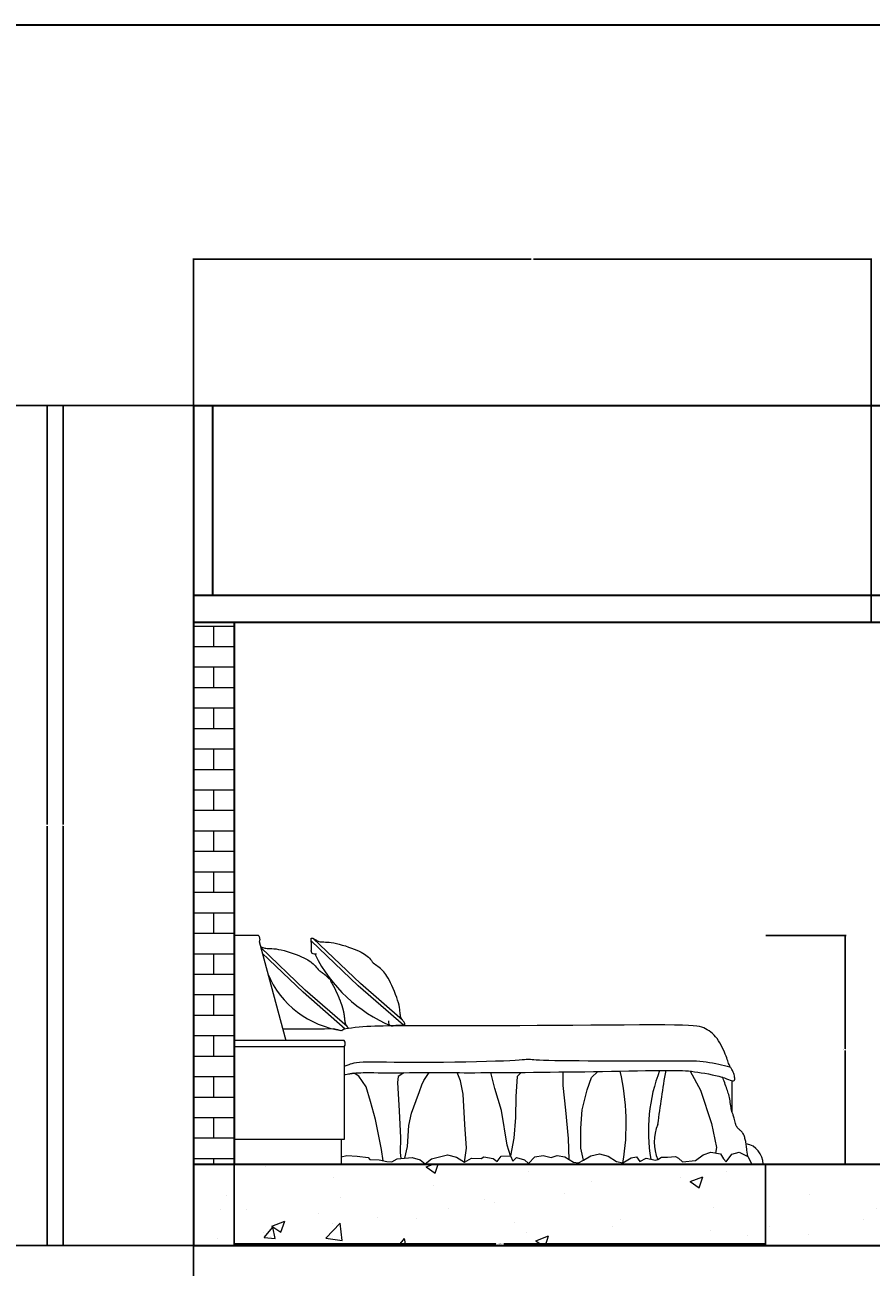
# Model space of a CAD drawing. Units: inches. Extents: x 2250 to 3547, y 1387 to 2604.
# Tile 7 of 11: x 2814 to 3002, y 2329 to 2604. Entities that reach past the tile are written whole.
import ezdxf

# ---------------------------------------------------------------- set-up
doc = ezdxf.new("R2010")
doc.units = ezdxf.units.IN
for name, color, linetype, lineweight in [('A-ANNO-DIMS', 2, 'Continuous', 18), ('A-ANNO-TTLB', 7, 'Continuous', 35), ('A-FLOR-PATT', 252, 'Continuous', 13), ('A-FURN', 9, 'Continuous', 18), ('A-SECT', 7, 'Continuous', 35), ('A-WALL-PATT', 252, 'Continuous', 13)]:
    doc.layers.add(name, color=color, linetype=linetype, lineweight=lineweight)
doc.styles.get("Standard").update_dxf_attribs({"font": 'arial.ttf'})
doc.dimstyles.get("Standard").update_dxf_attribs({"dimtxt": 0.18, "dimasz": 0.18, "dimexe": 0.18, "dimexo": 0.0625, "dimgap": 0.09, "dimtad": 0, "dimtih": 1, "dimtoh": 1, "dimdec": 4, "dimzin": 0, "dimdsep": 46, "dimtxsty": 'Standard', "dimcen": 0.09, "dimadec": 0, "dimazin": 0, "dimtfac": 1, "dimtdec": 4, "dimtofl": 0, "dimtmove": 0, "dimatfit": 3, "dimfxl": 1, "dimtolj": 1, "dimtzin": 0, "dimarcsym": 0})

# ---------------------------------------------------------------- blocks, each defined once
blk = doc.blocks.new('A$C08BC4B9A')
for p, q in [((0, 924.5), (0.5, 925)), ((0, 0), (0, 924.5)), ((95, 925), (0.5, 925)), ((101.1, 921.9), (105, 907.4)), ((311.4, 909.3), (311.5, 910.8)), ((311.5, 907.6), (311.4, 909.3)), ((311.5, 910.8), (311.7, 912.1)), ((311.7, 905.6), (311.5, 907.6)), ((311.7, 912.1), (312.1, 913.2)), ((312, 903.5), (311.7, 905.6)), ((312.1, 913.2), (312.7, 914.1)), ((312.7, 914.1), (313.6, 914.7)), ((313.6, 914.7), (314.7, 915)), ((314.7, 915), (316, 915.1)), ((316, 915.1), (317.6, 914.9)), ((317.6, 914.9), (319.3, 914.5)), ((319.3, 914.5), (321.1, 913.7)), ((511.6, 731.1), (320.5, 913.9)), ((321.1, 913.7), (323.2, 912.6)), ((323.2, 912.6), (325.4, 911.2)), ((325.4, 911.2), (327.8, 909.6)), ((327.8, 909.6), (330.4, 907.8)), ((330.4, 907.8), (333.3, 906.1)), ((333.3, 906.1), (336.4, 904.3)), ((101.4, 901.2), (208.9, 500)), ((106.6, 881.7), (106.8, 881.6)), ((106.8, 881.6), (109.7, 879.8)), ((288, 704.9), (107.8, 877.3)), ((109.7, 879.8), (112.8, 878.1)), ((112.8, 878.1), (116.3, 876.5)), ((116.3, 876.5), (120.1, 875.2)), ((120.1, 875.2), (124.3, 874.2)), ((124.3, 874.2), (128.9, 873.6)), ((128.9, 873.6), (134, 873.3)), ((134, 873.3), (139.6, 873.2)), ((139.6, 873.2), (146, 873)), ((146, 873), (153.1, 872.7)), ((153.1, 872.7), (161, 872.1)), ((161, 872.1), (169.8, 871.1)), ((169.8, 871.1), (179.7, 869.5)), ((179.7, 869.5), (190.6, 867.1)), ((190.6, 867.1), (202.3, 864.2)), ((202.3, 864.2), (214.5, 860.7)), ((214.5, 860.7), (226.9, 856.8)), ((226.9, 856.8), (239.3, 852.7)), ((502.9, 721.7), (311.9, 904.5)), ((312.3, 901.1), (312, 903.5)), ((312.6, 898.6), (312.3, 901.1)), ((312.9, 895.9), (312.6, 898.6)), ((312.7, 863.2), (312.8, 867.3)), ((313.1, 859.2), (312.7, 863.2)), ((312.8, 867.3), (313, 871.5)), ((313.1, 892.9), (312.9, 895.9)), ((313, 871.5), (313.3, 875.5)), ((313.3, 889.8), (313.1, 892.9)), ((314.3, 855.7), (313.1, 859.2)), ((313.4, 886.5), (313.3, 889.8)), ((313.3, 875.5), (313.4, 879.4)), ((313.4, 883), (313.4, 886.5)), ((313.4, 879.4), (313.4, 883)), ((316.7, 852.8), (314.3, 855.7)), ((336.4, 904.3), (339.9, 902.7)), ((339.9, 902.7), (343.7, 901.4)), ((343.7, 901.4), (347.9, 900.4)), ((347.9, 900.4), (352.5, 899.8)), ((352.5, 899.8), (357.6, 899.5)), ((357.6, 899.5), (363.2, 899.4)), ((363.2, 899.4), (369.6, 899.2)), ((369.6, 899.2), (376.7, 898.9)), ((376.7, 898.9), (384.6, 898.3)), ((384.6, 898.3), (393.4, 897.3)), ((393.4, 897.3), (403.3, 895.7)), ((403.3, 895.7), (414.2, 893.3)), ((414.2, 893.3), (425.9, 890.4)), ((425.9, 890.4), (438.1, 886.9)), ((438.1, 886.9), (450.5, 883.1)), ((450.5, 883.1), (462.9, 878.9)), ((462.9, 878.9), (474.9, 874.6)), ((474.9, 874.6), (486.3, 870.2)), ((486.3, 870.2), (496.8, 865.9)), ((496.8, 865.9), (506.1, 861.7)), ((506.1, 861.7), (514.3, 857.6)), ((514.3, 857.6), (521.6, 853.6)), ((279.2, 695.5), (114.2, 853.4)), ((239.3, 852.7), (251.3, 848.4)), ((251.3, 848.4), (262.7, 844)), ((262.7, 844), (273.2, 839.6)), ((273.2, 839.6), (282.5, 835.5)), ((282.5, 835.5), (290.7, 831.4)), ((290.7, 831.4), (298, 827.4)), ((298, 827.4), (304.4, 823.4)), ((304.4, 823.4), (310.1, 819.5)), ((310.1, 819.5), (315.2, 815.4)), ((315.2, 815.4), (319.8, 811.3)), ((320.4, 850.8), (316.7, 852.8)), ((319.8, 811.3), (324.1, 807)), ((325.8, 849.7), (320.4, 850.8)), ((324.1, 807), (328.1, 802.5)), ((333.2, 849.9), (325.8, 849.7)), ((521.6, 853.6), (528, 849.7)), ((528, 849.7), (533.7, 845.7)), ((533.7, 845.7), (538.8, 841.7)), ((538.8, 841.7), (543.4, 837.5)), ((543.4, 837.5), (547.7, 833.2)), ((547.7, 833.2), (551.7, 828.7)), ((551.7, 828.7), (555.6, 824.1)), ((555.6, 824.1), (559.4, 819.4)), ((559.4, 819.4), (563.3, 814.6)), ((563.3, 814.6), (567.7, 810.4)), ((572.2, 806.3), (567.7, 810.4)), ((577.3, 802.8), (572.2, 806.3)), ((328.1, 802.5), (332, 797.9)), ((332, 797.9), (335.8, 793.2)), ((335.8, 793.2), (339.7, 788.4)), ((339.7, 788.4), (344.1, 784.1)), ((344.2, 784), (344.1, 784.1)), ((344.5, 783.8), (344.2, 784)), ((344.9, 783.4), (344.5, 783.8)), ((345.5, 782.9), (344.9, 783.4)), ((346.1, 782.3), (345.5, 782.9)), ((346.8, 781.7), (346.1, 782.3)), ((347.6, 781.1), (346.8, 781.7)), ((348.3, 780.5), (347.6, 781.1)), ((349.1, 779.9), (348.3, 780.5)), ((349.8, 779.4), (349.1, 779.9)), ((350.5, 778.9), (349.8, 779.4)), ((351.1, 778.4), (350.5, 778.9)), ((351.8, 777.9), (351.1, 778.4)), ((352.4, 777.5), (351.8, 777.9)), ((353.1, 777), (352.4, 777.5)), ((353.7, 776.6), (353.1, 777)), ((354.3, 776.2), (353.7, 776.6)), ((354.9, 775.7), (354.3, 776.2)), ((355.6, 775.3), (354.9, 775.7)), ((356.2, 774.9), (355.6, 775.3)), ((356.8, 774.4), (356.2, 774.9)), ((357.4, 774), (356.8, 774.4)), ((358.1, 773.6), (357.4, 774)), ((358.7, 773.1), (358.1, 773.6)), ((359.3, 772.7), (358.7, 773.1)), ((359.9, 772.3), (359.3, 772.7)), ((360.5, 771.8), (359.9, 772.3)), ((361.2, 771.4), (360.5, 771.8)), ((361.8, 770.9), (361.2, 771.4)), ((362.4, 770.5), (361.8, 770.9)), ((363, 770), (362.4, 770.5)), ((363.6, 769.6), (363, 770)), ((364.2, 769.1), (363.6, 769.6)), ((364.8, 768.7), (364.2, 769.1)), ((365.4, 768.2), (364.8, 768.7)), ((366, 767.8), (365.4, 768.2)), ((366.6, 767.3), (366, 767.8)), ((367.2, 766.8), (366.6, 767.3)), ((367.8, 766.4), (367.2, 766.8)), ((368.3, 765.9), (367.8, 766.4)), ((368.9, 765.4), (368.3, 765.9)), ((369.5, 764.9), (368.9, 765.4)), ((370.1, 764.4), (369.5, 764.9)), ((370.7, 763.9), (370.1, 764.4)), ((371.2, 763.5), (370.7, 763.9)), ((371.8, 763), (371.2, 763.5)), ((372.4, 762.4), (371.8, 763)), ((373, 761.9), (372.4, 762.4)), ((373.5, 761.4), (373, 761.9)), ((374.1, 760.9), (373.5, 761.4)), ((374.7, 760.4), (374.1, 760.9)), ((375.2, 759.8), (374.7, 760.4)), ((375.8, 759.3), (375.2, 759.8)), ((376.3, 758.7), (375.8, 759.3)), ((376.9, 758.2), (376.3, 758.7)), ((377.4, 757.6), (376.9, 758.2)), ((378, 757), (377.4, 757.6)), ((378.6, 756.5), (378, 757)), ((379.2, 755.8), (378.6, 756.5)), ((379.8, 755.2), (379.2, 755.8)), ((380.5, 754.5), (379.8, 755.2)), ((381.3, 753.8), (380.5, 754.5)), ((582.3, 799.4), (577.3, 802.8)), ((587.2, 795.8), (582.3, 799.4)), ((592, 792.2), (587.2, 795.8)), ((596.6, 788.2), (592, 792.2)), ((601.1, 783.9), (596.6, 788.2)), ((605.5, 779.1), (601.1, 783.9)), ((609.9, 773.7), (605.5, 779.1)), ((614.3, 767.6), (609.9, 773.7)), ((618.8, 760.7), (614.3, 767.6)), ((623.5, 752.8), (618.8, 760.7)), ((457.7, 557), (288, 704.9)), ((382.2, 753.1), (381.3, 753.8)), ((383.2, 752.3), (382.2, 753.1)), ((384.2, 751.4), (383.2, 752.3)), ((385.4, 750.5), (384.2, 751.4)), ((386.6, 749.6), (385.4, 750.5)), ((387.8, 748.7), (386.6, 749.6)), ((388.9, 747.8), (387.8, 748.7)), ((389.9, 746.9), (388.9, 747.8)), ((390.8, 746), (389.9, 746.9)), ((391.4, 745.3), (390.8, 746)), ((391.9, 744.6), (391.4, 745.3)), ((392.1, 744), (391.9, 744.6)), ((392, 741.9), (392.1, 742.4)), ((392, 741.3), (392, 741.9)), ((392, 740.8), (392, 741.3)), ((392.1, 740.1), (392, 740.8)), ((392.2, 743.4), (392.1, 744)), ((392.1, 742.4), (392.2, 742.9)), ((392.4, 739.4), (392.1, 740.1)), ((392.2, 742.9), (392.2, 743.4)), ((392.7, 738.6), (392.4, 739.4)), ((393.1, 737.8), (392.7, 738.6)), ((393.6, 737), (393.1, 737.8)), ((394.1, 736.1), (393.6, 737)), ((394.7, 735.2), (394.1, 736.1)), ((395.2, 734.3), (394.7, 735.2)), ((395.8, 733.4), (395.2, 734.3)), ((396.4, 732.4), (395.8, 733.4)), ((397, 731.5), (396.4, 732.4)), ((397.6, 730.5), (397, 731.5)), ((398.2, 729.5), (397.6, 730.5)), ((398.7, 728.5), (398.2, 729.5)), ((399.3, 727.4), (398.7, 728.5)), ((399.9, 726.4), (399.3, 727.4)), ((400.5, 725.3), (399.9, 726.4)), ((401.1, 724.3), (400.5, 725.3)), ((401.7, 723.2), (401.1, 724.3)), ((402.4, 722), (401.7, 723.2)), ((403, 720.9), (402.4, 722)), ((403.6, 719.8), (403, 720.9)), ((404.2, 718.6), (403.6, 719.8)), ((404.8, 717.4), (404.2, 718.6)), ((405.4, 716.2), (404.8, 717.4)), ((406.1, 715), (405.4, 716.2)), ((406.7, 713.8), (406.1, 715)), ((407.3, 712.5), (406.7, 713.8)), ((408, 711.2), (407.3, 712.5)), ((408.6, 710), (408, 711.2)), ((409.3, 708.7), (408.6, 710)), ((409.9, 707.3), (409.3, 708.7)), ((410.6, 706), (409.9, 707.3)), ((411.2, 704.7), (410.6, 706)), ((411.9, 703.3), (411.2, 704.7)), ((685.7, 562.3), (502.9, 721.7)), ((681.3, 583.2), (511.6, 731.1)), ((628.4, 743.8), (623.5, 752.8)), ((633.5, 733.7), (628.4, 743.8)), ((638.7, 722.7), (633.5, 733.7)), ((643.9, 711), (638.7, 722.7)), ((649, 699), (643.9, 711)), ((450.1, 546.6), (279.2, 695.5)), ((412.5, 701.9), (411.9, 703.3)), ((413.2, 700.6), (412.5, 701.9)), ((413.8, 699.2), (413.2, 700.6)), ((414.5, 697.8), (413.8, 699.2)), ((415.1, 696.4), (414.5, 697.8)), ((415.8, 694.9), (415.1, 696.4)), ((416.4, 693.5), (415.8, 694.9)), ((417.1, 692.1), (416.4, 693.5)), ((417.7, 690.6), (417.1, 692.1)), ((418.4, 689.2), (417.7, 690.6)), ((419, 687.7), (418.4, 689.2)), ((419.7, 686.2), (419, 687.7)), ((420.3, 684.7), (419.7, 686.2)), ((421, 683.3), (420.3, 684.7)), ((421.6, 681.8), (421, 683.3)), ((422.2, 680.3), (421.6, 681.8)), ((422.9, 678.8), (422.2, 680.3)), ((423.5, 677.3), (422.9, 678.8)), ((424.1, 675.8), (423.5, 677.3)), ((424.7, 674.3), (424.1, 675.8)), ((425.4, 672.8), (424.7, 674.3)), ((426, 671.3), (425.4, 672.8)), ((426.6, 669.7), (426, 671.3)), ((427.2, 668.2), (426.6, 669.7)), ((427.8, 666.7), (427.2, 668.2)), ((428.4, 665.2), (427.8, 666.7)), ((429, 663.7), (428.4, 665.2)), ((429.6, 662.2), (429, 663.7)), ((430.1, 660.7), (429.6, 662.2)), ((430.7, 659.2), (430.1, 660.7)), ((431.3, 657.7), (430.7, 659.2)), ((431.8, 656.2), (431.3, 657.7)), ((432.4, 654.7), (431.8, 656.2)), ((432.9, 653.2), (432.4, 654.7)), ((653.8, 686.9), (649, 699)), ((658.2, 675), (653.8, 686.9)), ((662, 663.6), (658.2, 675)), ((665.2, 652.9), (662, 663.6)), ((433.4, 651.8), (432.9, 653.2)), ((434, 650.3), (433.4, 651.8)), ((434.5, 648.8), (434, 650.3)), ((435, 647.4), (434.5, 648.8)), ((435.5, 645.9), (435, 647.4)), ((436, 644.5), (435.5, 645.9)), ((436.5, 643.1), (436, 644.5)), ((436.9, 641.7), (436.5, 643.1)), ((437.4, 640.2), (436.9, 641.7)), ((437.9, 638.8), (437.4, 640.2)), ((438.3, 637.5), (437.9, 638.8)), ((438.7, 636.1), (438.3, 637.5)), ((439.1, 634.7), (438.7, 636.1)), ((439.6, 633.4), (439.1, 634.7)), ((440, 632), (439.6, 633.4)), ((440.3, 630.7), (440, 632)), ((440.7, 629.4), (440.3, 630.7)), ((441.1, 628.1), (440.7, 629.4)), ((441.4, 626.8), (441.1, 628.1)), ((441.8, 625.5), (441.4, 626.8)), ((442.1, 624.3), (441.8, 625.5)), ((442.4, 623.1), (442.1, 624.3)), ((442.7, 621.8), (442.4, 623.1)), ((443, 620.6), (442.7, 621.8)), ((443.3, 619.4), (443, 620.6)), ((443.6, 618.3), (443.3, 619.4)), ((443.8, 617.1), (443.6, 618.3)), ((444.1, 616), (443.8, 617.1)), ((444.3, 614.8), (444.1, 616)), ((444.5, 613.7), (444.3, 614.8)), ((444.7, 612.6), (444.5, 613.7)), ((445, 611.5), (444.7, 612.6)), ((445.2, 610.5), (445, 611.5)), ((445.4, 609.4), (445.2, 610.5)), ((445.5, 608.4), (445.4, 609.4)), ((445.7, 607.3), (445.5, 608.4)), ((445.9, 606.3), (445.7, 607.3)), ((446, 605.3), (445.9, 606.3)), ((446.2, 604.3), (446, 605.3)), ((446.4, 603.3), (446.2, 604.3)), ((667.5, 643.2), (665.2, 652.9)), ((669.2, 634.4), (667.5, 643.2)), ((670.4, 626.6), (669.2, 634.4)), ((671.3, 619.5), (670.4, 626.6)), ((671.9, 613.2), (671.3, 619.5)), ((672.5, 607.6), (671.9, 613.2)), ((673.1, 602.5), (672.5, 607.6)), ((446.5, 602.4), (446.4, 603.3)), ((446.6, 601.4), (446.5, 602.4)), ((446.8, 600.5), (446.6, 601.4)), ((446.9, 599.6), (446.8, 600.5)), ((447, 598.6), (446.9, 599.6)), ((447.1, 597.7), (447, 598.6)), ((447.2, 596.9), (447.1, 597.7)), ((447.3, 596), (447.2, 596.9)), ((447.4, 595.1), (447.3, 596)), ((447.5, 594.3), (447.4, 595.1)), ((447.6, 593.4), (447.5, 594.3)), ((447.7, 592.6), (447.6, 593.4)), ((447.8, 591.8), (447.7, 592.6)), ((447.9, 591), (447.8, 591.8)), ((448, 590.2), (447.9, 591)), ((448, 589.4), (448, 590.2)), ((448.1, 588.6), (448, 589.4)), ((448.2, 587.9), (448.1, 588.6)), ((448.3, 587.1), (448.2, 587.9)), ((448.3, 586.4), (448.3, 587.1)), ((448.4, 585.6), (448.3, 586.4)), ((448.5, 584.9), (448.4, 585.6)), ((448.6, 584.2), (448.5, 584.9)), ((448.6, 583.5), (448.6, 584.2)), ((448.7, 582.8), (448.6, 583.5)), ((448.8, 582.1), (448.7, 582.8)), ((448.9, 581.4), (448.8, 582.1)), ((448.9, 580.8), (448.9, 581.4)), ((449, 580.1), (448.9, 580.8)), ((449.1, 579.5), (449, 580.1)), ((449.2, 578.8), (449.1, 579.5)), ((449.3, 578.2), (449.2, 578.8)), ((449.4, 577.6), (449.3, 578.2)), ((449.5, 577), (449.4, 577.6)), ((449.6, 576.4), (449.5, 577)), ((449.7, 575.8), (449.6, 576.4)), ((449.8, 575.2), (449.7, 575.8)), ((449.9, 574.6), (449.8, 575.2)), ((450, 574), (449.9, 574.6)), ((450.1, 573.5), (450, 574)), ((450.3, 572.9), (450.1, 573.5)), ((450.4, 572.4), (450.3, 572.9)), ((450.5, 571.8), (450.4, 572.4)), ((450.7, 571.3), (450.5, 571.8)), ((450.8, 570.8), (450.7, 571.3)), ((451, 570.2), (450.8, 570.8)), ((451.1, 569.7), (451, 570.2)), ((451.3, 569.2), (451.1, 569.7)), ((451.5, 568.7), (451.3, 569.2)), ((451.6, 568.2), (451.5, 568.7)), ((451.8, 567.7), (451.6, 568.2)), ((452, 567.2), (451.8, 567.7)), ((452.2, 566.8), (452, 567.2)), ((452.4, 566.3), (452.2, 566.8)), ((452.6, 565.8), (452.4, 566.3)), ((452.8, 565.4), (452.6, 565.8)), ((453, 564.9), (452.8, 565.4)), ((453.2, 564.5), (453, 564.9)), ((453.4, 564), (453.2, 564.5)), ((453.6, 563.6), (453.4, 564)), ((453.8, 563.1), (453.6, 563.6)), ((454.1, 562.7), (453.8, 563.1)), ((454.3, 562.3), (454.1, 562.7)), ((454.5, 561.9), (454.3, 562.3)), ((454.8, 561.5), (454.5, 561.9)), ((455, 561.1), (454.8, 561.5)), ((455.2, 560.7), (455, 561.1)), ((455.5, 560.3), (455.2, 560.7)), ((455.7, 559.9), (455.5, 560.3)), ((456, 559.5), (455.7, 559.9)), ((456.2, 559.1), (456, 559.5)), ((456.4, 558.8), (456.2, 559.1)), ((456.7, 558.4), (456.4, 558.8)), ((456.9, 558), (456.7, 558.4)), ((457.2, 557.7), (456.9, 558)), ((457.4, 557.3), (457.2, 557.7)), ((457.7, 557), (457.4, 557.3)), ((457.9, 556.6), (457.7, 557)), ((458.2, 556.3), (457.9, 556.6)), ((458.4, 555.9), (458.2, 556.3)), ((458.7, 555.6), (458.4, 555.9)), ((458.9, 555.3), (458.7, 555.6)), ((459.2, 554.9), (458.9, 555.3)), ((459.4, 554.6), (459.2, 554.9)), ((459.7, 554.3), (459.4, 554.6)), ((459.9, 554), (459.7, 554.3)), ((460.2, 553.6), (459.9, 554)), ((460.4, 553.3), (460.2, 553.6)), ((460.7, 553), (460.4, 553.3)), ((506, 554.2), (490.5, 552.6)), ((521.7, 555.5), (506, 554.2)), ((537.6, 556.6), (521.7, 555.5)), ((553.6, 557.4), (537.6, 556.6)), ((569.7, 558.1), (553.6, 557.4)), ((586, 558.6), (569.7, 558.1)), ((603.2, 559), (586, 558.6)), ((621.8, 559.3), (603.2, 559)), ((642.6, 559.5), (621.8, 559.3)), ((624.8, 579.5), (625.2, 572.1)), ((625.2, 572.1), (626.6, 566.8)), ((626.6, 566.8), (629, 563.3)), ((629, 563.3), (632, 561.2)), ((632, 561.2), (635.6, 560.2)), ((635.6, 560.2), (639.6, 560.1)), ((639.6, 560.1), (643.7, 560.5)), ((666.5, 559.6), (642.6, 559.5)), ((643.7, 560.5), (647.9, 561)), ((647.9, 561), (651.9, 561.6)), ((651.9, 561.6), (655.7, 562)), ((655.7, 562), (659.3, 562.3)), ((659.3, 562.3), (662.8, 562.5)), ((662.8, 562.5), (666.1, 562.7)), ((666.1, 562.7), (669.2, 562.7)), ((693.9, 559.6), (666.5, 559.6)), ((669.2, 562.7), (672.2, 562.7)), ((672.2, 562.7), (674.9, 562.7)), ((674.1, 598), (673.1, 602.5)), ((675.4, 593.9), (674.1, 598)), ((674.9, 562.7), (677.5, 562.6)), ((677, 590.2), (675.4, 593.9)), ((678.8, 586.8), (677, 590.2)), ((677.5, 562.6), (679.8, 562.4)), ((680.8, 583.8), (678.8, 586.8)), ((679.8, 562.4), (682, 562.3)), ((682.8, 581.1), (680.8, 583.8)), ((682, 562.3), (683.9, 562.3)), ((684.7, 578.6), (682.8, 581.1)), ((683.9, 562.3), (685.7, 562.3)), ((686.5, 576.4), (684.7, 578.6)), ((685.7, 562.3), (687.2, 562.4)), ((688.1, 574.3), (686.5, 576.4)), ((687.2, 562.4), (688.5, 562.7)), ((689.3, 572.3), (688.1, 574.3)), ((688.5, 562.7), (689.5, 563.2)), ((690.2, 570.5), (689.3, 572.3)), ((689.5, 563.2), (690.3, 563.9)), ((690.8, 568.8), (690.2, 570.5)), ((690.3, 563.9), (690.9, 564.9)), ((691.1, 567.3), (690.8, 568.8)), ((690.9, 564.9), (691.1, 566)), ((691.1, 566), (691.1, 567.3)), ((725.8, 559.7), (693.9, 559.6)), ((762.8, 559.7), (725.8, 559.7)), ((805.4, 559.7), (762.8, 559.7)), ((853.4, 559.7), (805.4, 559.7)), ((906.2, 559.7), (853.4, 559.7)), ((963.4, 559.8), (906.2, 559.7)), ((1024.6, 559.9), (963.4, 559.8)), ((1089.2, 560.1), (1024.6, 559.9)), ((1156.7, 560.4), (1089.2, 560.1)), ((1226.8, 560.7), (1156.7, 560.4)), ((1298.7, 561.1), (1226.8, 560.7)), ((1371.2, 561.6), (1298.7, 561.1)), ((1443.1, 562.1), (1371.2, 561.6)), ((1512.8, 562.6), (1443.1, 562.1)), ((1579.1, 563), (1512.8, 562.6)), ((1640.5, 563.3), (1579.1, 563)), ((1695.8, 563.4), (1640.5, 563.3)), ((1743.5, 563.3), (1695.8, 563.4)), ((1782.8, 563), (1743.5, 563.3)), ((1814.2, 562.4), (1782.8, 563)), ((1838.9, 561.5), (1814.2, 562.4)), ((1858, 560.2), (1838.9, 561.5)), ((1872.6, 558.6), (1858, 560.2)), ((1883.7, 556.6), (1872.6, 558.6)), ((1892.6, 554.2), (1883.7, 556.6)), ((1900.3, 551.3), (1892.6, 554.2)), ((366.1, 546.8), (196.6, 546.1)), ((400.7, 547.5), (366.1, 546.8)), ((420, 543.6), (400.7, 547.5)), ((431.7, 540.1), (420, 543.6)), ((439.4, 542.5), (431.7, 540.1)), ((445.4, 545.7), (439.4, 542.5)), ((460.2, 548.4), (445.4, 545.7)), ((475.2, 550.7), (460.2, 548.4)), ((461, 552.6), (460.7, 553)), ((461.3, 552.3), (461, 552.6)), ((461.6, 551.9), (461.3, 552.3)), ((461.9, 551.5), (461.6, 551.9)), ((462.2, 551.1), (461.9, 551.5)), ((462.5, 550.7), (462.2, 551.1)), ((462.8, 550.3), (462.5, 550.7)), ((463.2, 549.8), (462.8, 550.3)), ((463.5, 549.4), (463.2, 549.8)), ((463.8, 548.9), (463.5, 549.4)), ((490.5, 552.6), (475.2, 550.7)), ((1907.7, 547.9), (1900.3, 551.3)), ((1915, 544), (1907.7, 547.9)), ((1922.1, 539.6), (1915, 544)), ((1929, 534.5), (1922.1, 539.6)), ((1935.8, 528.9), (1929, 534.5)), ((1942.3, 522.6), (1935.8, 528.9)), ((1948.6, 515.6), (1942.3, 522.6)), ((1954.6, 508), (1948.6, 515.6)), ((1960.4, 499.6), (1954.6, 508)), ((445.9, 500), (0, 500)), ((445.9, 475), (0, 475)), ((445.9, 475), (445.9, 100)), ((1965.8, 490.7), (1960.4, 499.6)), ((1970.9, 481.5), (1965.8, 490.7)), ((1975.6, 472.1), (1970.9, 481.5)), ((1980, 462.7), (1975.6, 472.1)), ((1984, 453.6), (1980, 462.7)), ((1987.5, 445), (1984, 453.6)), ((461.8, 402), (466.2, 403.7)), ((466.2, 403.7), (471.3, 405.6)), ((471.3, 405.6), (477.6, 407.5)), ((477.6, 407.5), (485.4, 409.4)), ((485.4, 409.4), (495.3, 411.1)), ((495.3, 411.1), (507.7, 412.5)), ((507.7, 412.5), (523, 413.5)), ((523, 413.5), (541.5, 414)), ((541.5, 414), (563.2, 414.2)), ((563.2, 414.2), (588.2, 414.1)), ((588.2, 414.1), (616.4, 413.7)), ((616.4, 413.7), (647.7, 413.3)), ((647.7, 413.3), (682, 412.9)), ((682, 412.9), (719.4, 412.6)), ((719.4, 412.6), (759.7, 412.4)), ((759.7, 412.4), (802.6, 412.6)), ((802.6, 412.6), (847.4, 413)), ((847.4, 413), (892.8, 413.6)), ((892.8, 413.6), (937.8, 414.4)), ((937.8, 414.4), (981.1, 415.3)), ((981.1, 415.3), (1021.7, 416.4)), ((1021.7, 416.4), (1058.6, 417.5)), ((1058.6, 417.5), (1090.4, 418.7)), ((1090.4, 418.7), (1116.5, 419.9)), ((1116.5, 419.9), (1137.2, 421)), ((1137.2, 421), (1153.4, 422.1)), ((1153.4, 422.1), (1165.7, 423)), ((1165.7, 423), (1174.9, 423.8)), ((1174.9, 423.8), (1181.7, 424.4)), ((1181.7, 424.4), (1186.9, 424.8)), ((1186.9, 424.8), (1191.2, 425)), ((1191.2, 425), (1195.4, 424.8)), ((1195.4, 424.8), (1200, 424.5)), ((1200, 424.5), (1205.8, 423.9)), ((1205.8, 423.9), (1213.3, 423.2)), ((1213.3, 423.2), (1223.1, 422.4)), ((1223.1, 422.4), (1236, 421.7)), ((1236, 421.7), (1252.5, 420.9)), ((1252.5, 420.9), (1273.3, 420.3)), ((1273.3, 420.3), (1298.7, 419.7)), ((1298.7, 419.7), (1328.3, 419.4)), ((1328.3, 419.4), (1361.1, 419.1)), ((1361.1, 419.1), (1396.4, 418.9)), ((1396.4, 418.9), (1433.4, 418.8)), ((1433.4, 418.8), (1471.3, 418.7)), ((1471.3, 418.7), (1509.3, 418.7)), ((1509.3, 418.7), (1546.6, 418.7)), ((1546.6, 418.7), (1582.4, 418.7)), ((1582.4, 418.7), (1616.7, 418.7)), ((1616.7, 418.7), (1649.3, 418.7)), ((1649.3, 418.7), (1680.1, 418.7)), ((1680.1, 418.7), (1709, 418.7)), ((1709, 418.7), (1736, 418.7)), ((1736, 418.7), (1760.9, 418.7)), ((1760.9, 418.7), (1783.8, 418.7)), ((1783.8, 418.7), (1804.5, 418.7)), ((1804.5, 418.7), (1823.2, 418.6)), ((1823.2, 418.6), (1840.3, 418.5)), ((1840.3, 418.5), (1856.1, 418.1)), ((1856.1, 418.1), (1870.7, 417.6)), ((1870.7, 417.6), (1884.5, 416.7)), ((1884.5, 416.7), (1897.8, 415.6)), ((1897.8, 415.6), (1910.8, 414)), ((1910.8, 414), (1923.7, 412)), ((1923.7, 412), (1936.5, 409.7)), ((1936.5, 409.7), (1949.1, 407.1)), ((1949.1, 407.1), (1961.3, 404.4)), ((1961.3, 404.4), (1973.1, 401.6)), ((1990.7, 437), (1987.5, 445)), ((1993.4, 429.7), (1990.7, 437)), ((1995.8, 423.3), (1993.4, 429.7)), ((1997.8, 417.5), (1995.8, 423.3)), ((1999.6, 412.4), (1997.8, 417.5)), ((2001.3, 407.8), (1999.6, 412.4)), ((2002.8, 403.7), (2001.3, 407.8)), ((2004.3, 400.1), (2002.8, 403.7)), ((445.9, 397.8), (449.1, 398.3)), ((445.9, 362), (481.5, 369.7)), ((445.9, 362.5), (450.4, 363.2)), ((449.1, 398.3), (453.4, 399.2)), ((450.4, 363.2), (457.2, 364.1)), ((453.4, 399.2), (457.6, 400.4)), ((457.2, 364.1), (463.4, 364.9)), ((457.6, 400.4), (461.8, 402)), ((463.4, 364.9), (468.9, 365.7)), ((468.9, 365.7), (473.6, 366.4)), ((473.6, 366.4), (477.6, 367.1)), ((477.6, 367.1), (481.1, 367.7)), ((481.1, 367.7), (484.4, 368.3)), ((484.4, 368.3), (488, 368.8)), ((504.7, 356.4), (486.2, 368.5)), ((488, 368.8), (492.3, 369.2)), ((492.3, 369.2), (497.5, 369.6)), ((497.5, 369.6), (504.1, 369.9)), ((504.1, 369.9), (512.5, 370.1)), ((534.3, 312.8), (504.7, 356.4)), ((512.5, 370.1), (522.9, 370.3)), ((522.9, 370.3), (535.3, 370.3)), ((535.3, 370.3), (549.5, 370.3)), ((549.5, 370.3), (565.4, 370.3)), ((565.4, 370.3), (582.8, 370.2)), ((582.8, 370.2), (601.6, 370.2)), ((601.6, 370.2), (621.6, 370.1)), ((621.6, 370.1), (642.7, 370.1)), ((642.7, 370.1), (664.7, 370.1)), ((663.6, 354.7), (661.8, 330.2)), ((687.3, 370.2), (663.6, 354.7)), ((664.7, 370.1), (687.3, 370.2)), ((687.3, 370.2), (710.4, 370.3)), ((710.4, 370.3), (733.4, 370.4)), ((733.4, 370.4), (756.3, 370.4)), ((756.3, 370.4), (778.7, 370.5)), ((768.3, 339), (789.4, 370.5)), ((778.7, 370.5), (800.2, 370.6)), ((800.2, 370.6), (820.7, 370.6)), ((820.7, 370.6), (840, 370.6)), ((840, 370.6), (858.3, 370.5)), ((858.3, 370.5), (876.2, 370.4)), ((876.2, 370.4), (894, 370.4)), ((894, 370.4), (912.3, 370.3)), ((916.7, 337.2), (903.2, 370.3)), ((912.3, 370.3), (931.5, 370.2)), ((931.5, 370.2), (952, 370.2)), ((952, 370.2), (974.3, 370.2)), ((974.3, 370.2), (998.7, 370.3)), ((998.7, 370.3), (1025.1, 370.4)), ((1025.1, 370.4), (1053.2, 370.6)), ((1054.7, 305.8), (1039.1, 370.5)), ((1053.2, 370.6), (1082.9, 370.8)), ((1082.9, 370.8), (1113.8, 371)), ((1113.8, 371), (1145.8, 371.3)), ((1145.5, 354.7), (1140.2, 274.4)), ((1162.2, 371.4), (1145.5, 354.7)), ((1145.8, 371.3), (1178.6, 371.6)), ((1178.6, 371.6), (1212, 371.9)), ((1212, 371.9), (1245.7, 372.2)), ((1245.7, 372.2), (1279.8, 372.6)), ((1279.8, 372.6), (1314.1, 373)), ((1314.1, 373), (1348.8, 373.4)), ((1332.3, 318), (1331.5, 373.2)), ((1348.8, 373.4), (1383.8, 373.8)), ((1383.8, 373.8), (1419.1, 374.3)), ((1419.1, 374.3), (1454.7, 374.8)), ((1445.8, 351.2), (1472.7, 375.1)), ((1454.7, 374.8), (1490.6, 375.4)), ((1490.6, 375.4), (1526.8, 376)), ((1526.8, 376), (1562.7, 376.6)), ((1562.7, 376.6), (1597.9, 377.2)), ((1597.9, 377.2), (1632, 377.8)), ((1632, 377.8), (1664.4, 378.4)), ((1664.4, 378.4), (1694.6, 378.9)), ((1694.6, 378.9), (1722.2, 379.3)), ((1722.2, 379.3), (1746.7, 379.5)), ((1746.7, 379.5), (1767.7, 379.7)), ((1767.7, 379.7), (1785.7, 379.6)), ((1785.7, 379.6), (1801.2, 379.4)), ((1801.2, 379.4), (1814.9, 378.9)), ((1814.9, 378.9), (1827.4, 378.2)), ((1827.4, 378.2), (1839.2, 377.2)), ((1839.2, 377.2), (1850.9, 375.9)), ((1845.1, 376.6), (1887, 298.9)), ((1850.9, 375.9), (1863.2, 374.3)), ((1863.2, 374.3), (1876.4, 372.4)), ((1876.4, 372.4), (1890.5, 370.2)), ((1890.5, 370.2), (1905, 367.7)), ((1905, 367.7), (1919.7, 364.9)), ((1919.7, 364.9), (1934.2, 362)), ((1934.2, 362), (1948.2, 358.9)), ((1948.2, 358.9), (1961.4, 355.7)), ((1961.4, 355.7), (1973.5, 352.4)), ((1973.1, 401.6), (1984.4, 398.8)), ((1973.5, 352.4), (1984.1, 349.1)), ((1977.1, 352.6), (1976.8, 353.5)), ((1978, 350), (1977.1, 352.6)), ((1984.4, 398.8), (1995, 396.1)), ((1995, 396.1), (2004.8, 393.6)), ((2005.8, 396.8), (2004.3, 400.1)), ((2007.5, 393.8), (2005.8, 396.8)), ((2009.2, 390.9), (2007.5, 393.8)), ((2010.9, 388.2), (2009.2, 390.9)), ((2012.7, 385.4), (2010.9, 388.2)), ((2014.5, 382.5), (2012.7, 385.4)), ((2016.4, 379.3), (2014.5, 382.5)), ((2018.2, 375.7), (2016.4, 379.3)), ((2020, 371.7), (2018.2, 375.7)), ((2021.7, 367.2), (2020, 371.7)), ((2023.2, 362.2), (2021.7, 367.2)), ((2024.6, 357.2), (2023.2, 362.2)), ((2025.5, 352.3), (2024.6, 357.2)), ((2026, 347.7), (2025.5, 352.3)), ((551.8, 253.5), (534.3, 312.8)), ((661.8, 330.2), (668.8, 215.1)), ((750.9, 293.6), (759.6, 321.5)), ((759.6, 321.5), (768.3, 339)), ((927.2, 283.1), (916.7, 337.2)), ((1082.6, 216.8), (1054.7, 305.8)), ((1342.8, 218.6), (1332.3, 318)), ((1428.3, 300.6), (1445.8, 351.2)), ((1979.4, 346.1), (1978, 350)), ((1981.2, 341.1), (1979.4, 346.1)), ((1983.2, 335.3), (1981.2, 341.1)), ((1985.5, 329), (1983.2, 335.3)), ((1984.1, 349.1), (1993.3, 345.9)), ((1987.8, 322.5), (1985.5, 329)), ((1990.1, 316.1), (1987.8, 322.5)), ((1992.3, 309.9), (1990.1, 316.1)), ((1994.4, 304), (1992.3, 309.9)), ((1993.3, 345.9), (2001.3, 342.9)), ((1996.4, 298.3), (1994.4, 304)), ((2001.3, 342.9), (2007.9, 340.5)), ((2007.9, 340.5), (2013.4, 338.6)), ((2013.4, 338.6), (2017.8, 337.5)), ((2015, 211.3), (2015, 338.2)), ((2017.8, 337.5), (2021.2, 337.3)), ((2021.2, 337.3), (2023.6, 338.3)), ((2023.6, 338.3), (2025.2, 340.5)), ((2025.2, 340.5), (2025.9, 343.7)), ((2025.9, 343.7), (2026, 347.7)), ((572.8, 180.2), (551.8, 253.5)), ((717.7, 206.4), (736.9, 257)), ((736.9, 257), (750.9, 293.6)), ((934.2, 161), (927.2, 283.1)), ((1140.2, 274.4), (1138.5, 188.9)), ((1409.1, 220.3), (1428.3, 300.6)), ((1887, 298.9), (1932.4, 164.5)), ((1998.2, 292.7), (1996.4, 298.3)), ((2000, 287.1), (1998.2, 292.7)), ((2001.6, 281.3), (2000, 287.1)), ((2003.1, 275.4), (2001.6, 281.3)), ((2004.5, 269.2), (2003.1, 275.4)), ((2005.8, 262.6), (2004.5, 269.2)), ((2006.9, 255.8), (2005.8, 262.6)), ((2008, 248.9), (2006.9, 255.8)), ((668.8, 215.1), (674, 106.9)), ((707.2, 155.8), (717.7, 206.4)), ((1105.3, 77.3), (1082.6, 216.8)), ((1353.2, 103.4), (1342.8, 218.6)), ((1403.9, 145.3), (1409.1, 220.3)), ((2009, 242.1), (2008, 248.9)), ((2010, 235.6), (2009, 242.1)), ((2011, 229.5), (2010, 235.6)), ((2011.9, 223.9), (2011, 229.5)), ((2012.9, 219), (2011.9, 223.9)), ((2013.9, 215), (2012.9, 219)), ((2014.9, 211.6), (2013.9, 215)), ((2015.9, 208.7), (2014.9, 211.6)), ((2017, 206), (2015.9, 208.7)), ((2018.1, 203.5), (2017, 206)), ((2019.2, 200.8), (2018.1, 203.5)), ((597.2, 59.8), (572.8, 180.2)), ((702, 72), (707.2, 155.8)), ((941.2, 65.1), (934.2, 161)), ((1138.5, 188.9), (1131.5, 105.2)), ((1932.4, 164.5), (1951.6, 66.8)), ((2020.3, 197.8), (2019.2, 200.8)), ((2021.4, 194.3), (2020.3, 197.8)), ((2022.5, 190.2), (2021.4, 194.3)), ((2023.7, 185.5), (2022.5, 190.2)), ((2024.9, 180.4), (2023.7, 185.5)), ((2026.1, 175.1), (2024.9, 180.4)), ((2027.4, 169.8), (2026.1, 175.1)), ((2028.9, 164.7), (2027.4, 169.8)), ((2030.5, 159.8), (2028.9, 164.7)), ((2032.2, 155.5), (2030.5, 159.8)), ((2034.1, 151.8), (2032.2, 155.5)), ((2036.1, 148.6), (2034.1, 151.8)), ((674, 106.9), (672.3, 47.6)), ((1131.5, 105.2), (1119, 34)), ((1356.3, 18.2), (1353.2, 103.4)), ((1403.9, 65.1), (1403.9, 145.3)), ((2038.3, 145.9), (2036.1, 148.6)), ((2040.5, 143.6), (2038.3, 145.9)), ((2042.8, 141.5), (2040.5, 143.6)), ((2045, 139.6), (2042.8, 141.5)), ((2047.3, 137.8), (2045, 139.6)), ((2049.5, 136), (2047.3, 137.8)), ((2051.6, 134.1), (2049.5, 136)), ((2053.6, 132), (2051.6, 134.1)), ((2055.6, 129.7), (2053.6, 132)), ((2057.4, 127.3), (2055.6, 129.7)), ((2059.1, 124.7), (2057.4, 127.3)), ((2060.8, 121.9), (2059.1, 124.7)), ((2062.3, 118.9), (2060.8, 121.9)), ((2063.8, 115.6), (2062.3, 118.9)), ((2065.1, 112), (2063.8, 115.6)), ((2066.4, 108.3), (2065.1, 112)), ((2067.5, 104.3), (2066.4, 108.3)), ((2068.6, 100.2), (2067.5, 104.3)), ((445.9, 100), (0, 100)), ((433.9, 100), (433.9, 0)), ((602.8, 13.7), (597.2, 59.8)), ((690.4, 23.9), (702, 72)), ((932.8, 7.5), (941.2, 65.1)), ((1119, 34), (1105.3, 77.3)), ((1414.2, 16.7), (1403.9, 65.1)), ((1951.6, 66.8), (1948.4, 44.8)), ((2069.5, 95.9), (2068.6, 100.2)), ((2070.4, 91.5), (2069.5, 95.9)), ((2071.2, 87), (2070.4, 91.5)), ((2072, 82.5), (2071.2, 87)), ((2072.6, 77.9), (2072, 82.5)), ((2073.3, 73.2), (2072.6, 77.9)), ((2073.9, 68.1), (2073.3, 73.2)), ((2074.7, 62.4), (2073.9, 68.1)), ((2075.5, 56), (2074.7, 62.4)), ((2076.5, 48.7), (2075.5, 56)), ((0, 0), (2150.5, 0)), ((433.9, 29.5), (455.7, 35.6)), ((455.7, 35.6), (497.9, 32.5)), ((497.9, 32.5), (543.3, 26.2)), ((543.3, 26.2), (549.6, 18.4)), ((549.6, 18.4), (587.1, 16.9)), ((587.1, 16.9), (618.4, 10.6)), ((618.4, 10.6), (638.7, 9)), ((638.7, 9), (660.6, 21.5)), ((660.6, 21.5), (720.1, 26.2)), ((672.3, 47.6), (674.3, 22.6)), ((720.1, 26.2), (752.9, 16.9)), ((752.9, 16.9), (773.3, 1.2)), ((773.3, 1.2), (798.3, 21.5)), ((798.3, 21.5), (864, 37.2)), ((864, 37.2), (900, 27.8)), ((900, 27.8), (932.8, 7.5)), ((932.8, 7.5), (961, 24.7)), ((961, 24.7), (1000.1, 23.1)), ((1000.1, 23.1), (1011.1, 29.4)), ((1011.1, 29.4), (1048.6, 23.1)), ((1048.6, 23.1), (1064.3, 10.6)), ((1064.3, 10.6), (1081.5, 32.5)), ((1081.5, 32.5), (1119, 34)), ((1119, 34), (1128.4, 12.2)), ((1128.4, 12.2), (1142.5, 26.2)), ((1142.5, 26.2), (1175.3, 16.9)), ((1175.3, 16.9), (1191, 2.8)), ((1191, 2.8), (1217.6, 29.4)), ((1217.6, 29.4), (1250.4, 35.6)), ((1250.4, 35.6), (1283.3, 26.2)), ((1283.3, 26.2), (1307.8, 35.4)), ((1307.8, 35.4), (1339.1, 29.2)), ((1339.1, 29.2), (1373.5, 7.3)), ((1373.5, 7.3), (1393.8, 5.7)), ((1393.8, 5.7), (1414.2, 16.7)), ((1414.2, 16.7), (1443.9, 33.9)), ((1443.9, 33.9), (1478.3, 41.7)), ((1478.3, 41.7), (1514.3, 32.3)), ((1514.3, 32.3), (1547.2, 10.4)), ((1547.2, 10.4), (1573.7, 5.7)), ((1573.7, 5.7), (1606.6, 26.1)), ((1606.6, 26.1), (1628.5, 29.2)), ((1628.5, 29.2), (1642.6, 10.4)), ((1642.6, 10.4), (1667.6, 24.5)), ((1667.6, 24.5), (1705.2, 16.7)), ((1705.2, 16.7), (1714.5, 18.2)), ((1714.5, 18.2), (1730.2, 27.6)), ((1730.2, 27.6), (1745.8, 27.6)), ((1745.8, 27.6), (1753.7, 27.6)), ((1753.7, 27.6), (1786.5, 30.7)), ((1786.5, 30.7), (1799, 24.5)), ((1799, 24.5), (1814.7, 8.9)), ((1814.7, 8.9), (1867.9, 15.1)), ((1867.9, 15.1), (1897.6, 37)), ((1897.6, 37), (1928.9, 47.9)), ((1928.9, 47.9), (1968, 41.7)), ((1968, 41.7), (1980.5, 21.4)), ((1980.5, 21.4), (1991.4, 8.9)), ((1991.4, 8.9), (2014.9, 40.1)), ((2014.9, 40.1), (2044.6, 47.9)), ((2044.6, 47.9), (2079, 30.7)), ((2077.6, 40.3), (2076.5, 48.7)), ((2079, 30.7), (2077.6, 40.3)), ((2079, 30.7), (2095.6, 0))]:
    blk.add_line(p, q)
for centre, radius, start, end in [((96.2, 920.6), 5, 15, 105), ((100.1, 906.1), 5, 285, 15), ((863.9, 1112.1), 597.2, 206.2473, 247.5264), ((487.1, 917.9), 380.4, 202.7795, 262.4477), ((429, 487.5), 21, 323.3696, 36.6304), ((634, 163.3), 952.9, 350.4806, 12.9339), ((2353.4, 135.1), 676.8, 158.8487, 189.7401), ((6455, -433.2), 4778, 170.2062, 172.8555), ((1887.2, 90.1), 187, 157.7155, 202.6016), ((2056.3, 0.1), 84.2, 359.9053, 78.7345)]:
    blk.add_arc(centre, radius, start, end)
blk = doc.blocks.new('*D38')
at = {"layer": 'A-ANNO-DIMS', "color": 0, "lineweight": -2, "transparency": 16777216}
for p, q in [((2860.63, 2351.89), (2860.63, 2334.13)), ((2978.25, 2351.89), (2978.25, 2334.13)), ((2860.81, 2334.31), (2918.55, 2334.31)), ((2978.07, 2334.31), (2920.33, 2334.31))]:
    blk.add_line(p, q, dxfattribs=at)
at = {"layer": 'A-ANNO-DIMS', "color": 0, "transparency": 16777216}
for points in [[(2860.81, 2334.34), (2860.81, 2334.28), (2860.63, 2334.31)], [(2978.07, 2334.34), (2978.07, 2334.28), (2978.25, 2334.31)]]:
    blk.add_solid(points, dxfattribs=at)
at = {"layer": 'Defpoints', "color": 0, "transparency": 16777216}
for p in [(2860.63, 2351.95), (2978.25, 2351.95), (2978.25, 2334.31)]:
    blk.add_point(p, dxfattribs=at)
at = {"layer": 'A-ANNO-DIMS', "color": 0, "transparency": 16777216, "insert": (2919.44, 2334.31), "char_height": 0.18, "attachment_point": 5}
blk.add_mtext('\\A1;BED 118 TYP.', dxfattribs=at)
blk = doc.blocks.new('*D39')
at = {"layer": 'A-ANNO-DIMS', "color": 0, "lineweight": -2, "transparency": 16777216}
for p, q in [((2978.31, 2402.6), (2996.07, 2402.6)), ((2995.89, 2402.42), (2995.89, 2377.46)), ((2995.89, 2352.13), (2995.89, 2377.09)), ((2978.31, 2351.95), (2996.07, 2351.95))]:
    blk.add_line(p, q, dxfattribs=at)
at = {"layer": 'A-ANNO-DIMS', "color": 0, "transparency": 16777216}
for points in [[(2995.86, 2402.42), (2995.92, 2402.42), (2995.89, 2402.6)], [(2995.86, 2352.13), (2995.92, 2352.13), (2995.89, 2351.95)]]:
    blk.add_solid(points, dxfattribs=at)
at = {"layer": 'Defpoints', "color": 0, "transparency": 16777216}
for p in [(2978.25, 2402.6), (2995.89, 2402.6), (2978.25, 2351.95)]:
    blk.add_point(p, dxfattribs=at)
at = {"layer": 'A-ANNO-DIMS', "color": 0, "transparency": 16777216, "insert": (2995.89, 2377.28), "char_height": 0.18, "attachment_point": 5}
blk.add_mtext('\\A1;51 TYP.', dxfattribs=at)
blk = doc.blocks.new('*D96')
at = {"layer": 'A-ANNO-DIMS', "color": 0, "lineweight": -2, "transparency": 16777216}
for p, q in [((2798.6, 2519.95), (2822.97, 2519.95)), ((2822.79, 2519.77), (2822.79, 2427.13)), ((2822.79, 2334.13), (2822.79, 2426.77)), ((2774.6, 2333.95), (2822.97, 2333.95))]:
    blk.add_line(p, q, dxfattribs=at)
at = {"layer": 'A-ANNO-DIMS', "color": 0, "transparency": 16777216}
for points in [[(2822.76, 2519.77), (2822.82, 2519.77), (2822.79, 2519.95)], [(2822.76, 2334.13), (2822.82, 2334.13), (2822.79, 2333.95)]]:
    blk.add_solid(points, dxfattribs=at)
at = {"layer": 'Defpoints', "color": 0, "transparency": 16777216}
for p in [(2798.54, 2519.95), (2822.79, 2519.95), (2774.54, 2333.95)]:
    blk.add_point(p, dxfattribs=at)
at = {"layer": 'A-ANNO-DIMS', "color": 0, "transparency": 16777216, "insert": (2822.79, 2426.95), "char_height": 0.18, "attachment_point": 5}
blk.add_mtext('\\A1;186', dxfattribs=at)
blk = doc.blocks.new('*D108')
at = {"layer": 'A-ANNO-DIMS', "color": 0, "lineweight": -2, "transparency": 16777216}
for p, q in [((2851.63, 2333.89), (2851.63, 2251.45)), ((3283.63, 2333.89), (3283.63, 2251.45)), ((2851.81, 2251.63), (3067.34, 2251.63)), ((3283.45, 2251.63), (3067.92, 2251.63))]:
    blk.add_line(p, q, dxfattribs=at)
at = {"layer": 'A-ANNO-DIMS', "color": 0, "transparency": 16777216}
for points in [[(2851.81, 2251.66), (2851.81, 2251.6), (2851.63, 2251.63)], [(3283.45, 2251.66), (3283.45, 2251.6), (3283.63, 2251.63)]]:
    blk.add_solid(points, dxfattribs=at)
at = {"layer": 'Defpoints', "color": 0, "transparency": 16777216}
for p in [(2851.63, 2333.95), (3283.63, 2333.95), (3283.63, 2251.63)]:
    blk.add_point(p, dxfattribs=at)
at = {"layer": 'A-ANNO-DIMS', "color": 0, "transparency": 16777216, "insert": (3067.63, 2251.63), "char_height": 0.18, "attachment_point": 5}
blk.add_mtext('\\A1;432', dxfattribs=at)
blk = doc.blocks.new('*D109')
at = {"layer": 'A-ANNO-DIMS', "color": 0, "lineweight": -2, "transparency": 16777216}
for p, q in [((2851.57, 2519.95), (2819.1, 2519.95)), ((2819.28, 2519.77), (2819.28, 2427.13)), ((2819.28, 2334.13), (2819.28, 2426.77)), ((2851.57, 2333.95), (2819.1, 2333.95))]:
    blk.add_line(p, q, dxfattribs=at)
at = {"layer": 'A-ANNO-DIMS', "color": 0, "transparency": 16777216}
for points in [[(2819.25, 2519.77), (2819.31, 2519.77), (2819.28, 2519.95)], [(2819.25, 2334.13), (2819.31, 2334.13), (2819.28, 2333.95)]]:
    blk.add_solid(points, dxfattribs=at)
at = {"layer": 'Defpoints', "color": 0, "transparency": 16777216}
for p in [(2819.28, 2519.95), (2851.63, 2519.95), (2851.63, 2333.95)]:
    blk.add_point(p, dxfattribs=at)
at = {"layer": 'A-ANNO-DIMS', "color": 0, "transparency": 16777216, "insert": (2819.28, 2426.95), "char_height": 0.18, "attachment_point": 5}
blk.add_mtext('\\A1;186', dxfattribs=at)
blk = doc.blocks.new('*D110')
at = {"layer": 'A-ANNO-DIMS', "color": 0, "lineweight": -2, "transparency": 16777216}
for p, q in [((2851.63, 2520.01), (2851.63, 2552.48)), ((2851.81, 2552.3), (2926.35, 2552.3)), ((3001.45, 2552.3), (2926.91, 2552.3)), ((3001.63, 2472.01), (3001.63, 2552.48))]:
    blk.add_line(p, q, dxfattribs=at)
at = {"layer": 'A-ANNO-DIMS', "color": 0, "transparency": 16777216}
for points in [[(2851.81, 2552.33), (2851.81, 2552.27), (2851.63, 2552.3)], [(3001.45, 2552.33), (3001.45, 2552.27), (3001.63, 2552.3)]]:
    blk.add_solid(points, dxfattribs=at)
at = {"layer": 'Defpoints', "color": 0, "transparency": 16777216}
for p in [(3001.63, 2552.3), (2851.63, 2519.95), (3001.63, 2471.95)]:
    blk.add_point(p, dxfattribs=at)
at = {"layer": 'A-ANNO-DIMS', "color": 0, "transparency": 16777216, "insert": (2926.63, 2552.3), "char_height": 0.18, "attachment_point": 5}
blk.add_mtext('\\A1;150', dxfattribs=at)

msp = doc.modelspace()

# ---------------------------------------------------------------- hatches: boundary and pattern name
at = {"layer": 'A-FLOR-PATT'}
h = msp.add_hatch(dxfattribs=at)
h.set_pattern_fill('AR-CONC', color=256, scale=0.16, style=0)
h.paths.add_polyline_path([(2851.6288, 2333.9493), (3283.6288, 2333.9493), (3283.6288, 2351.9493), (2851.6288, 2351.9493)])
at = {"layer": 'A-WALL-PATT'}
h = msp.add_hatch(dxfattribs=at)
h.set_pattern_fill('AR-BRSTD', color=256, scale=0.0669322, style=0)
h.paths.add_polyline_path([(2851.6288, 2351.9493), (2860.6288, 2351.9493), (2860.6288, 2471.9493), (2851.6288, 2471.9493)])

# ---------------------------------------------------------------- linework, layer by layer
at = {"layer": 'A-ANNO-TTLB'}
msp.add_lwpolyline([(2250.1093, 2604.1988), (3546.995, 2604.1988), (3546.995, 1386.7251), (2250.1093, 1386.7251)], close=True, dxfattribs=at)
at = {"layer": 'A-SECT'}
for p, q in [((2851.6288, 2519.9493), (2851.6288, 2333.9493)), ((2851.6288, 2519.9493), (3283.6288, 2519.9493)), ((2855.9125, 2477.9493), (2855.9125, 2519.9493)), ((2851.6288, 2477.9493), (3283.6288, 2477.9493)), ((2851.6288, 2471.9493), (3283.6288, 2471.9493)), ((2860.6288, 2471.9493), (2860.6288, 2351.9493)), ((2851.6288, 2351.9493), (3283.6288, 2351.9493)), ((2851.6288, 2333.9493), (3283.6288, 2333.9493))]:
    msp.add_line(p, q, dxfattribs=at)

# ---------------------------------------------------------------- block references
at = {"layer": 'A-FURN', "xscale": 0.0546942147408242, "yscale": 0.0546942147408242, "zscale": 0.0546942147408242}
msp.add_blockref('A$C08BC4B9A', (2860.6288, 2351.9493), dxfattribs=at)

# ---------------------------------------------------------------- dimensions: what is measured, and where the dimension line sits
at = {"layer": 'A-ANNO-DIMS'}
for base, p1, p2, picture, middle in [((3001.6288, 2552.2993), (2851.6288, 2519.9493), (3001.6288, 2471.9493), '*D110', (2926.6288, 2552.2993)), ((3283.6288, 2251.631), (2851.6288, 2333.9493), (3283.6288, 2333.9493), '*D108', (3067.6288, 2251.631))]:
    dim = msp.add_linear_dim(base=base, p1=p1, p2=p2, dimstyle='Standard', override={"dimdec": 0, "dimlfac": 1, "dimrnd": 0, "dimzin": 0, "dimdsep": 46, "dimlunit": 2}, dxfattribs=at)
    dim.commit()
    dim.dimension.update_dxf_attribs({"geometry": picture, "text_midpoint": middle})
for base, p1, p2, picture, middle in [((2822.7878, 2519.9493), (2774.5378, 2333.9493), (2798.5378, 2519.9493), '*D96', (2822.7878, 2426.9493)), ((2819.2788, 2519.9493), (2851.6288, 2333.9493), (2851.6288, 2519.9493), '*D109', (2819.2788, 2426.9493))]:
    dim = msp.add_linear_dim(base=base, p1=p1, p2=p2, angle=90, dimstyle='Standard', override={"dimdec": 0, "dimlfac": 1, "dimrnd": 0, "dimzin": 0, "dimdsep": 46, "dimlunit": 2}, dxfattribs=at)
    dim.commit()
    dim.dimension.update_dxf_attribs({"geometry": picture, "text_midpoint": middle})
dim = msp.add_linear_dim(base=(2995.8894, 2402.602), p1=(2978.2467, 2351.9493), p2=(2978.2467, 2402.602), angle=90, text='<> TYP.', dimstyle='Standard', override={"dimdec": 0, "dimlfac": 1, "dimrnd": 0, "dimzin": 0, "dimdsep": 46, "dimlunit": 2}, dxfattribs=at)
dim.commit()
dim.dimension.update_dxf_attribs({"geometry": '*D39', "text_midpoint": (2995.8894, 2377.2757)})
dim = msp.add_linear_dim(base=(2978.2467, 2334.3066), p1=(2860.6288, 2351.9493), p2=(2978.2467, 2351.9493), text='BED <> TYP.', dimstyle='Standard', override={"dimdec": 0, "dimlfac": 1, "dimrnd": 0, "dimzin": 0, "dimdsep": 46, "dimlunit": 2}, dxfattribs=at)
dim.commit()
dim.dimension.update_dxf_attribs({"geometry": '*D38', "text_midpoint": (2919.4377, 2334.3066)})

doc.saveas('drawing.dxf')
